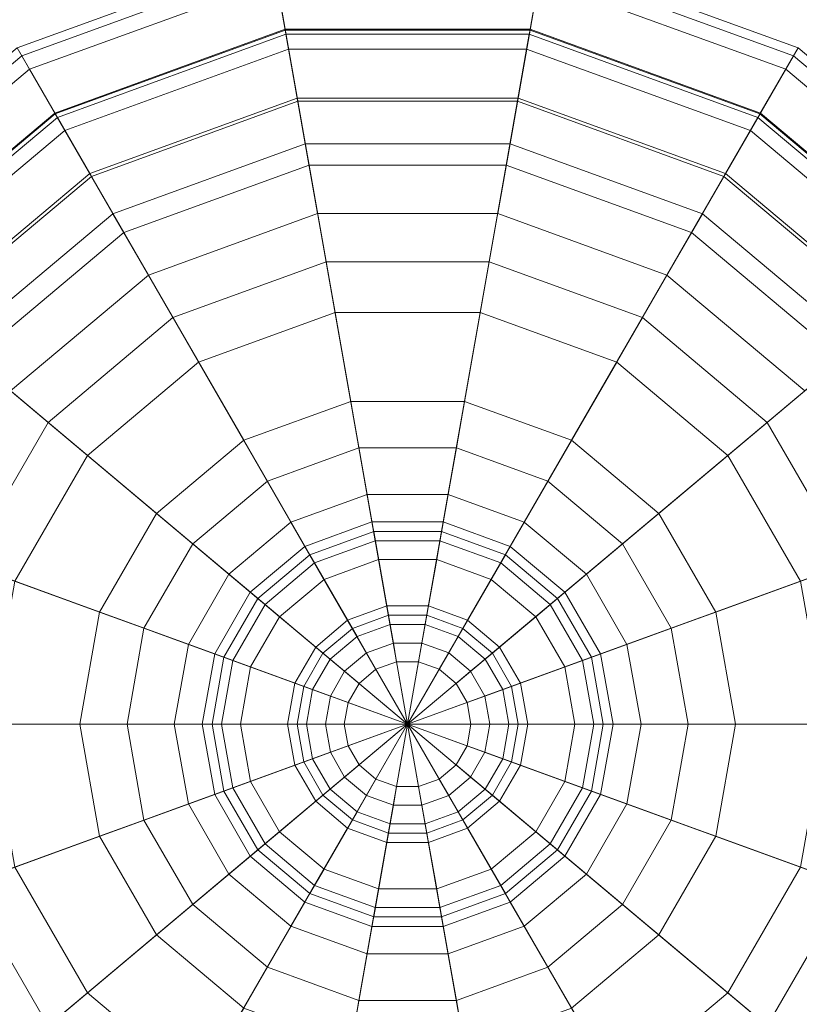
# Model space of a CAD drawing. Units: inches. Extents: x 375 to 1122, y 27 to 1069.
# Tile 32 of 155: x 732.389 to 733.741, y 280.756 to 282.464. Entities that reach past the tile are written whole.
import ezdxf

# ---------------------------------------------------------------- set-up
doc = ezdxf.new("R2010")
doc.units = ezdxf.units.IN
doc.layers.add('A-ANNO-DIMS', color=2, linetype='Continuous', lineweight=18)
doc.layers.add('Furniture', color=30, linetype='Continuous', lineweight=18)
doc.styles.get("Standard").update_dxf_attribs({"font": 'arial.ttf'})
doc.dimstyles.new('ISO-25', dxfattribs={"dimtxt": 12, "dimasz": 2.5, "dimexe": 1.5, "dimexo": 1.5, "dimtad": 1, "dimdec": 1, "dimlunit": 3, "dimtxsty": 'Standard', "dimblk": 'ARCHTICK', "dimcen": 2.5, "dimadec": 0, "dimazin": 0, "dimtfac": 1, "dimtdec": 1, "dimtmove": 0, "dimatfit": 3, "dimfxl": 1.5, "dimfxlon": 1, "dimarcsym": 0})

# ---------------------------------------------------------------- blocks, each defined once
blk = doc.blocks.new('A$C403C54AD')
for points in [[(1.626464, 1.23678, -0.04658), (1.626464, 1.202917, -0.043501), (1.626464, 1.202917, -0.043501), (1.614883, 1.234737, -0.04658)], [(1.638046, 1.234737, -0.04658), (1.626464, 1.202917, -0.043501), (1.626464, 1.202917, -0.043501), (1.626464, 1.23678, -0.04658)], [(1.614883, 1.234737, -0.04658), (1.626464, 1.202917, -0.043501), (1.626464, 1.202917, -0.043501), (1.604698, 1.228857, -0.04658)], [(1.64823, 1.228857, -0.04658), (1.626464, 1.202917, -0.043501), (1.626464, 1.202917, -0.043501), (1.638046, 1.234737, -0.04658)], [(1.626464, 1.217132, -0.040074), (1.626464, 1.233514, -0.043349), (1.616, 1.231669, -0.043349), (1.621603, 1.216274, -0.040074)], [(1.631326, 1.216274, -0.040074), (1.636929, 1.231669, -0.043349), (1.626464, 1.233514, -0.043349), (1.626464, 1.217132, -0.040074)], [(1.621603, 1.216274, -0.040074), (1.616, 1.231669, -0.043349), (1.606797, 1.226356, -0.043349), (1.617327, 1.213806, -0.040074)], [(1.635601, 1.213806, -0.040074), (1.646131, 1.226356, -0.043349), (1.636929, 1.231669, -0.043349), (1.631326, 1.216274, -0.040074)], [(1.604698, 1.228857, -0.04658), (1.626464, 1.202917, -0.043501), (1.626464, 1.202917, -0.043501), (1.597139, 1.219849, -0.04658)], [(1.606797, 1.226356, -0.043349), (1.604698, 1.228857, -0.04658), (1.597139, 1.219849, -0.04658), (1.599967, 1.218216, -0.043349)], [(1.65579, 1.219849, -0.04658), (1.626464, 1.202917, -0.043501), (1.626464, 1.202917, -0.043501), (1.64823, 1.228857, -0.04658)], [(1.606823, 1.226325, 0.116404), (1.604954, 1.228552, 0.10318), (1.597484, 1.219649, 0.10318), (1.600002, 1.218195, 0.116404)], [(1.604954, 1.228552, 0.10318), (1.605388, 1.228035, 0.074938), (1.598069, 1.219312, 0.074938), (1.597484, 1.219649, 0.10318)], [(1.617085, 1.228687, 0.056929), (1.619501, 1.222047, 0.046697), (1.613379, 1.218512, 0.046697), (1.608836, 1.223925, 0.056929)], [(1.644092, 1.223925, 0.056929), (1.63955, 1.218512, 0.046697), (1.633427, 1.222047, 0.046697), (1.635844, 1.228687, 0.056929)], [(1.605388, 1.228035, 0.074938), (1.608836, 1.223925, 0.056929), (1.602714, 1.216629, 0.056929), (1.598069, 1.219312, 0.074938)], [(1.617327, 1.213806, -0.040074), (1.606797, 1.226356, -0.043349), (1.599967, 1.218216, -0.043349), (1.614154, 1.210025, -0.040074)], [(1.610035, 1.222497, 0.12581), (1.606823, 1.226325, 0.116404), (1.600002, 1.218195, 0.116404), (1.604329, 1.215697, 0.12581)], [(1.606937, 1.226189, 0.102963), (1.608743, 1.224037, 0.115599), (1.602589, 1.216702, 0.115599), (1.600155, 1.218107, 0.102963)], [(1.60736, 1.225685, 0.075423), (1.606937, 1.226189, 0.102963), (1.600155, 1.218107, 0.102963), (1.600725, 1.217778, 0.075423)], [(1.638774, 1.210025, -0.040074), (1.652961, 1.218216, -0.043349), (1.646131, 1.226356, -0.043349), (1.635601, 1.213806, -0.040074)], [(1.620264, 1.219951, 0.048884), (1.618046, 1.226046, 0.058276), (1.610643, 1.221772, 0.058276), (1.614812, 1.216804, 0.048884)], [(1.638116, 1.216804, 0.048884), (1.642285, 1.221772, 0.058276), (1.634882, 1.226046, 0.058276), (1.632664, 1.219951, 0.048884)], [(1.610643, 1.221772, 0.058276), (1.60736, 1.225685, 0.075423), (1.600725, 1.217778, 0.075423), (1.605149, 1.215224, 0.058276)], [(1.608743, 1.224037, 0.115599), (1.612014, 1.220139, 0.12581), (1.606995, 1.214158, 0.12581), (1.602589, 1.216702, 0.115599)], [(1.608836, 1.223925, 0.056929), (1.613379, 1.218512, 0.046697), (1.608834, 1.213096, 0.046697), (1.602714, 1.216629, 0.056929)], [(1.626464, 1.223275, 0.046697), (1.626464, 1.213036, 0.03933), (1.623003, 1.212426, 0.03933), (1.619501, 1.222047, 0.046697)], [(1.633427, 1.222047, 0.046697), (1.629925, 1.212426, 0.03933), (1.626464, 1.213036, 0.03933), (1.626464, 1.223275, 0.046697)], [(1.612014, 1.220139, 0.12581), (1.610035, 1.222497, 0.12581), (1.604329, 1.215697, 0.12581), (1.606995, 1.214158, 0.12581)], [(1.619501, 1.222047, 0.046697), (1.623003, 1.212426, 0.03933), (1.61996, 1.210669, 0.03933), (1.613379, 1.218512, 0.046697)], [(1.63955, 1.218512, 0.046697), (1.632968, 1.210669, 0.03933), (1.629925, 1.212426, 0.03933), (1.633427, 1.222047, 0.046697)], [(1.614812, 1.216804, 0.048884), (1.610643, 1.221772, 0.058276), (1.605149, 1.215224, 0.058276), (1.610766, 1.211981, 0.048884)], [(1.642163, 1.211981, 0.048884), (1.64778, 1.215224, 0.058276), (1.642285, 1.221772, 0.058276), (1.638116, 1.216804, 0.048884)], [(1.626464, 1.211822, 0.042248), (1.626464, 1.221045, 0.048884), (1.620264, 1.219951, 0.048884), (1.623419, 1.211285, 0.042248)], [(1.62951, 1.211285, 0.042248), (1.632664, 1.219951, 0.048884), (1.626464, 1.221045, 0.048884), (1.626464, 1.211822, 0.042248)], [(1.597139, 1.219849, -0.04658), (1.626464, 1.202917, -0.043501), (1.626464, 1.202917, -0.043501), (1.593116, 1.208798, -0.04658)], [(1.599967, 1.218216, -0.043349), (1.597139, 1.219849, -0.04658), (1.593116, 1.208798, -0.04658), (1.596333, 1.20823, -0.043349)], [(1.623419, 1.211285, 0.042248), (1.620264, 1.219951, 0.048884), (1.614812, 1.216804, 0.048884), (1.620741, 1.209738, 0.042248)], [(1.659812, 1.208798, -0.04658), (1.626464, 1.202917, -0.043501), (1.626464, 1.202917, -0.043501), (1.65579, 1.219849, -0.04658)], [(1.632188, 1.209738, 0.042248), (1.638116, 1.216804, 0.048884), (1.632664, 1.219951, 0.048884), (1.62951, 1.211285, 0.042248)], [(1.600002, 1.218195, 0.116404), (1.597484, 1.219649, 0.10318), (1.593509, 1.208728, 0.10318), (1.596372, 1.208223, 0.116404)], [(1.597484, 1.219649, 0.10318), (1.598069, 1.219312, 0.074938), (1.594174, 1.208611, 0.074938), (1.593509, 1.208728, 0.10318)], [(1.598069, 1.219312, 0.074938), (1.602714, 1.216629, 0.056929), (1.599457, 1.20768, 0.056929), (1.594174, 1.208611, 0.074938)], [(1.613379, 1.218512, 0.046697), (1.61996, 1.210669, 0.03933), (1.617701, 1.207977, 0.03933), (1.608834, 1.213096, 0.046697)], [(1.644094, 1.213096, 0.046697), (1.635227, 1.207977, 0.03933), (1.632968, 1.210669, 0.03933), (1.63955, 1.218512, 0.046697)], [(1.614154, 1.210025, -0.040074), (1.599967, 1.218216, -0.043349), (1.596333, 1.20823, -0.043349), (1.612466, 1.205386, -0.040074)], [(1.604329, 1.215697, 0.12581), (1.600002, 1.218195, 0.116404), (1.596372, 1.208223, 0.116404), (1.601293, 1.207356, 0.12581)], [(1.600155, 1.218107, 0.102963), (1.602589, 1.216702, 0.115599), (1.599314, 1.207705, 0.115599), (1.596547, 1.208193, 0.102963)], [(1.600725, 1.217778, 0.075423), (1.600155, 1.218107, 0.102963), (1.596547, 1.208193, 0.102963), (1.597195, 1.208078, 0.075423)], [(1.605149, 1.215224, 0.058276), (1.600725, 1.217778, 0.075423), (1.597195, 1.208078, 0.075423), (1.602225, 1.207191, 0.058276)], [(1.620741, 1.209738, 0.042248), (1.614812, 1.216804, 0.048884), (1.610766, 1.211981, 0.048884), (1.618753, 1.207369, 0.042248)], [(1.626464, 1.215084, -0.037209), (1.626464, 1.217132, -0.040074), (1.621603, 1.216274, -0.040074), (1.622303, 1.21435, -0.037209)], [(1.630625, 1.21435, -0.037209), (1.631326, 1.216274, -0.040074), (1.626464, 1.217132, -0.040074), (1.626464, 1.215084, -0.037209)], [(1.634175, 1.207369, 0.042248), (1.642163, 1.211981, 0.048884), (1.638116, 1.216804, 0.048884), (1.632188, 1.209738, 0.042248)], [(1.602589, 1.216702, 0.115599), (1.606995, 1.214158, 0.12581), (1.604324, 1.206821, 0.12581), (1.599314, 1.207705, 0.115599)], [(1.602714, 1.216629, 0.056929), (1.608834, 1.213096, 0.046697), (1.606416, 1.206452, 0.046697), (1.599457, 1.20768, 0.056929)], [(1.622303, 1.21435, -0.037209), (1.621603, 1.216274, -0.040074), (1.617327, 1.213806, -0.040074), (1.618644, 1.212238, -0.037209)], [(1.634285, 1.212238, -0.037209), (1.635601, 1.213806, -0.040074), (1.631326, 1.216274, -0.040074), (1.630625, 1.21435, -0.037209)], [(1.606995, 1.214158, 0.12581), (1.604329, 1.215697, 0.12581), (1.601293, 1.207356, 0.12581), (1.604324, 1.206821, 0.12581)], [(1.610766, 1.211981, 0.048884), (1.605149, 1.215224, 0.058276), (1.602225, 1.207191, 0.058276), (1.608612, 1.206065, 0.048884)], [(1.626464, 1.210988, -0.035163), (1.626464, 1.215084, -0.037209), (1.622303, 1.21435, -0.037209), (1.623704, 1.210502, -0.035163)], [(1.629225, 1.210502, -0.035163), (1.630625, 1.21435, -0.037209), (1.626464, 1.215084, -0.037209), (1.626464, 1.210988, -0.035163)], [(1.623704, 1.210502, -0.035163), (1.622303, 1.21435, -0.037209), (1.618644, 1.212238, -0.037209), (1.621276, 1.2091, -0.035163)], [(1.631652, 1.2091, -0.035163), (1.634285, 1.212238, -0.037209), (1.630625, 1.21435, -0.037209), (1.629225, 1.210502, -0.035163)], [(1.618644, 1.212238, -0.037209), (1.617327, 1.213806, -0.040074), (1.614154, 1.210025, -0.040074), (1.615928, 1.209001, -0.037209)], [(1.637001, 1.209001, -0.037209), (1.638774, 1.210025, -0.040074), (1.635601, 1.213806, -0.040074), (1.634285, 1.212238, -0.037209)], [(1.608834, 1.213096, 0.046697), (1.617701, 1.207977, 0.03933), (1.616499, 1.204675, 0.03933), (1.606416, 1.206452, 0.046697)], [(1.626464, 1.213036, 0.03933), (1.626464, 1.208122, 0.038511), (1.624684, 1.207808, 0.038511), (1.623003, 1.212426, 0.03933)], [(1.629925, 1.212426, 0.03933), (1.628244, 1.207808, 0.038511), (1.626464, 1.208122, 0.038511), (1.626464, 1.213036, 0.03933)], [(1.646512, 1.206452, 0.046697), (1.636429, 1.204675, 0.03933), (1.635227, 1.207977, 0.03933), (1.644094, 1.213096, 0.046697)], [(1.621276, 1.2091, -0.035163), (1.618644, 1.212238, -0.037209), (1.615928, 1.209001, -0.037209), (1.619474, 1.206953, -0.035163)], [(1.623003, 1.212426, 0.03933), (1.624684, 1.207808, 0.038511), (1.623119, 1.206904, 0.038511), (1.61996, 1.210669, 0.03933)], [(1.632968, 1.210669, 0.03933), (1.629809, 1.206904, 0.038511), (1.628244, 1.207808, 0.038511), (1.629925, 1.212426, 0.03933)], [(1.633454, 1.206953, -0.035163), (1.637001, 1.209001, -0.037209), (1.634285, 1.212238, -0.037209), (1.631652, 1.2091, -0.035163)], [(1.618753, 1.207369, 0.042248), (1.610766, 1.211981, 0.048884), (1.608612, 1.206065, 0.048884), (1.617695, 1.204464, 0.042248)], [(1.626464, 1.202917, 0.040765), (1.626464, 1.211822, 0.042248), (1.623419, 1.211285, 0.042248), (1.626464, 1.202917, 0.040765)], [(1.626464, 1.202917, 0.040765), (1.62951, 1.211285, 0.042248), (1.626464, 1.211822, 0.042248), (1.626464, 1.202917, 0.040765)], [(1.635233, 1.204464, 0.042248), (1.644316, 1.206065, 0.048884), (1.642163, 1.211981, 0.048884), (1.634175, 1.207369, 0.042248)], [(1.626464, 1.202917, 0.040765), (1.623419, 1.211285, 0.042248), (1.620741, 1.209738, 0.042248), (1.626464, 1.202917, 0.040765)], [(1.626464, 1.211398, 0.035646), (1.626464, 1.207302, 0.033599), (1.624964, 1.207038, 0.033599), (1.623564, 1.210887, 0.035646)], [(1.626464, 1.210169, 0.037692), (1.626464, 1.211398, 0.035646), (1.623564, 1.210887, 0.035646), (1.623984, 1.209732, 0.037692)], [(1.629365, 1.210887, 0.035646), (1.627964, 1.207038, 0.033599), (1.626464, 1.207302, 0.033599), (1.626464, 1.211398, 0.035646)], [(1.628944, 1.209732, 0.037692), (1.629365, 1.210887, 0.035646), (1.626464, 1.211398, 0.035646), (1.626464, 1.210169, 0.037692)], [(1.626464, 1.202917, 0.040765), (1.632188, 1.209738, 0.042248), (1.62951, 1.211285, 0.042248), (1.626464, 1.202917, 0.040765)], [(1.623564, 1.210887, 0.035646), (1.624964, 1.207038, 0.033599), (1.623646, 1.206277, 0.033599), (1.621013, 1.209414, 0.035646)], [(1.623984, 1.209732, 0.037692), (1.623564, 1.210887, 0.035646), (1.621013, 1.209414, 0.035646), (1.621803, 1.208473, 0.037692)], [(1.626464, 1.207712, -0.029842), (1.626464, 1.210988, -0.035163), (1.623704, 1.210502, -0.035163), (1.624824, 1.207423, -0.029842)], [(1.628104, 1.207423, -0.029842), (1.629225, 1.210502, -0.035163), (1.626464, 1.210988, -0.035163), (1.626464, 1.207712, -0.029842)], [(1.631915, 1.209414, 0.035646), (1.629283, 1.206277, 0.033599), (1.627964, 1.207038, 0.033599), (1.629365, 1.210887, 0.035646)], [(1.631126, 1.208473, 0.037692), (1.631915, 1.209414, 0.035646), (1.629365, 1.210887, 0.035646), (1.628944, 1.209732, 0.037692)], [(1.61996, 1.210669, 0.03933), (1.623119, 1.206904, 0.038511), (1.621957, 1.205519, 0.038511), (1.617701, 1.207977, 0.03933)], [(1.624824, 1.207423, -0.029842), (1.623704, 1.210502, -0.035163), (1.621276, 1.2091, -0.035163), (1.623382, 1.20659, -0.029842)], [(1.629546, 1.20659, -0.029842), (1.631652, 1.2091, -0.035163), (1.629225, 1.210502, -0.035163), (1.628104, 1.207423, -0.029842)], [(1.635227, 1.207977, 0.03933), (1.630971, 1.205519, 0.038511), (1.629809, 1.206904, 0.038511), (1.632968, 1.210669, 0.03933)], [(1.615928, 1.209001, -0.037209), (1.614154, 1.210025, -0.040074), (1.612466, 1.205386, -0.040074), (1.614482, 1.20503, -0.037209)], [(1.626464, 1.208122, 0.038511), (1.626464, 1.210169, 0.037692), (1.623984, 1.209732, 0.037692), (1.624684, 1.207808, 0.038511)], [(1.628244, 1.207808, 0.038511), (1.628944, 1.209732, 0.037692), (1.626464, 1.210169, 0.037692), (1.626464, 1.208122, 0.038511)], [(1.638446, 1.20503, -0.037209), (1.640462, 1.205386, -0.040074), (1.638774, 1.210025, -0.040074), (1.637001, 1.209001, -0.037209)], [(1.626464, 1.202917, 0.040765), (1.620741, 1.209738, 0.042248), (1.618753, 1.207369, 0.042248), (1.626464, 1.202917, 0.040765)], [(1.624684, 1.207808, 0.038511), (1.623984, 1.209732, 0.037692), (1.621803, 1.208473, 0.037692), (1.623119, 1.206904, 0.038511)], [(1.626464, 1.202917, 0.040765), (1.634175, 1.207369, 0.042248), (1.632188, 1.209738, 0.042248), (1.626464, 1.202917, 0.040765)], [(1.629809, 1.206904, 0.038511), (1.631126, 1.208473, 0.037692), (1.628944, 1.209732, 0.037692), (1.628244, 1.207808, 0.038511)], [(1.621013, 1.209414, 0.035646), (1.623646, 1.206277, 0.033599), (1.622667, 1.20511, 0.033599), (1.61912, 1.207158, 0.035646)], [(1.621803, 1.208473, 0.037692), (1.621013, 1.209414, 0.035646), (1.61912, 1.207158, 0.035646), (1.620184, 1.206543, 0.037692)], [(1.623382, 1.20659, -0.029842), (1.621276, 1.2091, -0.035163), (1.619474, 1.206953, -0.035163), (1.622312, 1.205315, -0.029842)], [(1.633809, 1.207158, 0.035646), (1.630262, 1.20511, 0.033599), (1.629283, 1.206277, 0.033599), (1.631915, 1.209414, 0.035646)], [(1.630616, 1.205315, -0.029842), (1.633454, 1.206953, -0.035163), (1.631652, 1.2091, -0.035163), (1.629546, 1.20659, -0.029842)], [(1.632744, 1.206543, 0.037692), (1.633809, 1.207158, 0.035646), (1.631915, 1.209414, 0.035646), (1.631126, 1.208473, 0.037692)], [(1.593116, 1.208798, -0.04658), (1.626464, 1.202917, -0.043501), (1.626464, 1.202917, -0.043501), (1.593116, 1.197037, -0.04658)], [(1.596333, 1.20823, -0.043349), (1.593116, 1.208798, -0.04658), (1.593116, 1.197037, -0.04658), (1.596333, 1.197604, -0.043349)], [(1.596372, 1.208223, 0.116404), (1.593509, 1.208728, 0.10318), (1.593509, 1.197107, 0.10318), (1.596372, 1.197611, 0.116404)], [(1.619474, 1.206953, -0.035163), (1.615928, 1.209001, -0.037209), (1.614482, 1.20503, -0.037209), (1.618516, 1.204319, -0.035163)], [(1.659812, 1.197037, -0.04658), (1.626464, 1.202917, -0.043501), (1.626464, 1.202917, -0.043501), (1.659812, 1.208798, -0.04658)], [(1.634413, 1.204319, -0.035163), (1.638446, 1.20503, -0.037209), (1.637001, 1.209001, -0.037209), (1.633454, 1.206953, -0.035163)], [(1.594174, 1.208611, 0.074938), (1.599457, 1.20768, 0.056929), (1.599457, 1.198155, 0.056929), (1.594174, 1.197224, 0.074938)], [(1.623119, 1.206904, 0.038511), (1.621803, 1.208473, 0.037692), (1.620184, 1.206543, 0.037692), (1.621957, 1.205519, 0.038511)], [(1.630971, 1.205519, 0.038511), (1.632744, 1.206543, 0.037692), (1.631126, 1.208473, 0.037692), (1.629809, 1.206904, 0.038511)], [(1.612466, 1.205386, -0.040074), (1.596333, 1.20823, -0.043349), (1.596333, 1.197604, -0.043349), (1.612466, 1.200449, -0.040074)], [(1.601293, 1.207356, 0.12581), (1.596372, 1.208223, 0.116404), (1.596372, 1.197611, 0.116404), (1.601293, 1.198479, 0.12581)], [(1.596547, 1.208193, 0.102963), (1.599314, 1.207705, 0.115599), (1.599314, 1.19813, 0.115599), (1.596547, 1.197642, 0.102963)], [(1.597195, 1.208078, 0.075423), (1.596547, 1.208193, 0.102963), (1.596547, 1.197642, 0.102963), (1.597195, 1.197756, 0.075423)], [(1.602225, 1.207191, 0.058276), (1.597195, 1.208078, 0.075423), (1.597195, 1.197756, 0.075423), (1.602225, 1.198643, 0.058276)], [(1.617701, 1.207977, 0.03933), (1.621957, 1.205519, 0.038511), (1.621339, 1.203821, 0.038511), (1.616499, 1.204675, 0.03933)], [(1.636429, 1.204675, 0.03933), (1.631589, 1.203821, 0.038511), (1.630971, 1.205519, 0.038511), (1.635227, 1.207977, 0.03933)], [(1.599314, 1.207705, 0.115599), (1.604324, 1.206821, 0.12581), (1.604324, 1.199014, 0.12581), (1.599314, 1.19813, 0.115599)], [(1.599457, 1.20768, 0.056929), (1.606416, 1.206452, 0.046697), (1.606416, 1.199382, 0.046697), (1.599457, 1.198155, 0.056929)], [(1.625245, 1.206268, -0.021247), (1.624824, 1.207423, -0.029842), (1.623382, 1.20659, -0.029842), (1.624172, 1.205649, -0.021247)], [(1.626464, 1.206483, -0.021247), (1.626464, 1.207712, -0.029842), (1.624824, 1.207423, -0.029842), (1.625245, 1.206268, -0.021247)], [(1.627684, 1.206268, -0.021247), (1.628104, 1.207423, -0.029842), (1.626464, 1.207712, -0.029842), (1.626464, 1.206483, -0.021247)], [(1.628756, 1.205649, -0.021247), (1.629546, 1.20659, -0.029842), (1.628104, 1.207423, -0.029842), (1.627684, 1.206268, -0.021247)], [(1.604324, 1.206821, 0.12581), (1.601293, 1.207356, 0.12581), (1.601293, 1.198479, 0.12581), (1.604324, 1.199014, 0.12581)], [(1.608612, 1.206065, 0.048884), (1.602225, 1.207191, 0.058276), (1.602225, 1.198643, 0.058276), (1.608612, 1.19977, 0.048884)], [(1.626464, 1.202917, 0.040765), (1.618753, 1.207369, 0.042248), (1.617695, 1.204464, 0.042248), (1.626464, 1.202917, 0.040765)], [(1.61912, 1.207158, 0.035646), (1.622667, 1.20511, 0.033599), (1.622146, 1.203679, 0.033599), (1.618112, 1.20439, 0.035646)], [(1.620184, 1.206543, 0.037692), (1.61912, 1.207158, 0.035646), (1.618112, 1.20439, 0.035646), (1.619322, 1.204177, 0.037692)], [(1.622312, 1.205315, -0.029842), (1.619474, 1.206953, -0.035163), (1.618516, 1.204319, -0.035163), (1.621742, 1.20375, -0.029842)], [(1.624964, 1.207038, 0.033599), (1.625525, 1.205499, 0.027051), (1.624699, 1.205022, 0.027051), (1.623646, 1.206277, 0.033599)], [(1.626464, 1.207302, 0.033599), (1.626464, 1.205664, 0.027051), (1.625525, 1.205499, 0.027051), (1.624964, 1.207038, 0.033599)], [(1.626464, 1.202917, 0.040765), (1.635233, 1.204464, 0.042248), (1.634175, 1.207369, 0.042248), (1.626464, 1.202917, 0.040765)], [(1.627964, 1.207038, 0.033599), (1.627404, 1.205499, 0.027051), (1.626464, 1.205664, 0.027051), (1.626464, 1.207302, 0.033599)], [(1.629283, 1.206277, 0.033599), (1.62823, 1.205022, 0.027051), (1.627404, 1.205499, 0.027051), (1.627964, 1.207038, 0.033599)], [(1.634816, 1.20439, 0.035646), (1.630783, 1.203679, 0.033599), (1.630262, 1.20511, 0.033599), (1.633809, 1.207158, 0.035646)], [(1.631186, 1.20375, -0.029842), (1.634413, 1.204319, -0.035163), (1.633454, 1.206953, -0.035163), (1.630616, 1.205315, -0.029842)], [(1.633606, 1.204177, 0.037692), (1.634816, 1.20439, 0.035646), (1.633809, 1.207158, 0.035646), (1.632744, 1.206543, 0.037692)], [(1.621957, 1.205519, 0.038511), (1.620184, 1.206543, 0.037692), (1.619322, 1.204177, 0.037692), (1.621339, 1.203821, 0.038511)], [(1.624172, 1.205649, -0.021247), (1.623382, 1.20659, -0.029842), (1.622312, 1.205315, -0.029842), (1.623376, 1.2047, -0.021247)], [(1.629552, 1.2047, -0.021247), (1.630616, 1.205315, -0.029842), (1.629546, 1.20659, -0.029842), (1.628756, 1.205649, -0.021247)], [(1.631589, 1.203821, 0.038511), (1.633606, 1.204177, 0.037692), (1.632744, 1.206543, 0.037692), (1.630971, 1.205519, 0.038511)], [(1.606416, 1.206452, 0.046697), (1.616499, 1.204675, 0.03933), (1.616499, 1.20116, 0.03933), (1.606416, 1.199382, 0.046697)], [(1.623646, 1.206277, 0.033599), (1.624699, 1.205022, 0.027051), (1.624085, 1.204291, 0.027051), (1.622667, 1.20511, 0.033599)], [(1.625525, 1.205499, 0.027051), (1.625245, 1.206268, -0.021247), (1.624172, 1.205649, -0.021247), (1.624699, 1.205022, 0.027051)], [(1.626464, 1.205664, 0.027051), (1.626464, 1.206483, -0.021247), (1.625245, 1.206268, -0.021247), (1.625525, 1.205499, 0.027051)], [(1.627404, 1.205499, 0.027051), (1.627684, 1.206268, -0.021247), (1.626464, 1.206483, -0.021247), (1.626464, 1.205664, 0.027051)], [(1.62823, 1.205022, 0.027051), (1.628756, 1.205649, -0.021247), (1.627684, 1.206268, -0.021247), (1.627404, 1.205499, 0.027051)], [(1.630262, 1.20511, 0.033599), (1.628843, 1.204291, 0.027051), (1.62823, 1.205022, 0.027051), (1.629283, 1.206277, 0.033599)], [(1.646512, 1.199382, 0.046697), (1.636429, 1.20116, 0.03933), (1.636429, 1.204675, 0.03933), (1.646512, 1.206452, 0.046697)], [(1.617695, 1.204464, 0.042248), (1.608612, 1.206065, 0.048884), (1.608612, 1.19977, 0.048884), (1.617695, 1.201371, 0.042248)], [(1.635233, 1.201371, 0.042248), (1.644316, 1.19977, 0.048884), (1.644316, 1.206065, 0.048884), (1.635233, 1.204464, 0.042248)], [(1.614482, 1.20503, -0.037209), (1.612466, 1.205386, -0.040074), (1.612466, 1.200449, -0.040074), (1.614482, 1.200805, -0.037209)], [(1.623376, 1.2047, -0.021247), (1.622312, 1.205315, -0.029842), (1.621742, 1.20375, -0.029842), (1.622952, 1.203537, -0.021247)], [(1.624699, 1.205022, 0.027051), (1.624172, 1.205649, -0.021247), (1.623376, 1.2047, -0.021247), (1.624085, 1.204291, 0.027051)], [(1.628843, 1.204291, 0.027051), (1.629552, 1.2047, -0.021247), (1.628756, 1.205649, -0.021247), (1.62823, 1.205022, 0.027051)], [(1.629976, 1.203537, -0.021247), (1.631186, 1.20375, -0.029842), (1.630616, 1.205315, -0.029842), (1.629552, 1.2047, -0.021247)], [(1.638446, 1.200805, -0.037209), (1.640462, 1.200449, -0.040074), (1.640462, 1.205386, -0.040074), (1.638446, 1.20503, -0.037209)], [(1.618516, 1.204319, -0.035163), (1.614482, 1.20503, -0.037209), (1.614482, 1.200805, -0.037209), (1.618516, 1.201516, -0.035163)], [(1.622667, 1.20511, 0.033599), (1.624085, 1.204291, 0.027051), (1.623759, 1.203394, 0.027051), (1.622146, 1.203679, 0.033599)], [(1.630783, 1.203679, 0.033599), (1.629169, 1.203394, 0.027051), (1.628843, 1.204291, 0.027051), (1.630262, 1.20511, 0.033599)], [(1.634413, 1.201516, -0.035163), (1.638446, 1.200805, -0.037209), (1.638446, 1.20503, -0.037209), (1.634413, 1.204319, -0.035163)], [(1.616499, 1.204675, 0.03933), (1.621339, 1.203821, 0.038511), (1.621339, 1.202014, 0.038511), (1.616499, 1.20116, 0.03933)], [(1.626464, 1.202917, 0.040765), (1.617695, 1.204464, 0.042248), (1.617695, 1.201371, 0.042248), (1.626464, 1.202917, 0.040765)], [(1.618112, 1.20439, 0.035646), (1.622146, 1.203679, 0.033599), (1.622146, 1.202156, 0.033599), (1.618112, 1.201445, 0.035646)], [(1.619322, 1.204177, 0.037692), (1.618112, 1.20439, 0.035646), (1.618112, 1.201445, 0.035646), (1.619322, 1.201658, 0.037692)], [(1.624085, 1.204291, 0.027051), (1.623376, 1.2047, -0.021247), (1.622952, 1.203537, -0.021247), (1.623759, 1.203394, 0.027051)], [(1.626464, 1.202917, 0.040765), (1.635233, 1.201371, 0.042248), (1.635233, 1.204464, 0.042248), (1.626464, 1.202917, 0.040765)], [(1.629169, 1.203394, 0.027051), (1.629976, 1.203537, -0.021247), (1.629552, 1.2047, -0.021247), (1.628843, 1.204291, 0.027051)], [(1.634816, 1.201445, 0.035646), (1.630783, 1.202156, 0.033599), (1.630783, 1.203679, 0.033599), (1.634816, 1.20439, 0.035646)], [(1.636429, 1.20116, 0.03933), (1.631589, 1.202014, 0.038511), (1.631589, 1.203821, 0.038511), (1.636429, 1.204675, 0.03933)], [(1.633606, 1.201658, 0.037692), (1.634816, 1.201445, 0.035646), (1.634816, 1.20439, 0.035646), (1.633606, 1.204177, 0.037692)], [(1.621742, 1.20375, -0.029842), (1.618516, 1.204319, -0.035163), (1.618516, 1.201516, -0.035163), (1.621742, 1.202085, -0.029842)], [(1.621339, 1.203821, 0.038511), (1.619322, 1.204177, 0.037692), (1.619322, 1.201658, 0.037692), (1.621339, 1.202014, 0.038511)], [(1.631186, 1.202085, -0.029842), (1.634413, 1.201516, -0.035163), (1.634413, 1.204319, -0.035163), (1.631186, 1.20375, -0.029842)], [(1.631589, 1.202014, 0.038511), (1.633606, 1.201658, 0.037692), (1.633606, 1.204177, 0.037692), (1.631589, 1.203821, 0.038511)], [(1.622952, 1.203537, -0.021247), (1.621742, 1.20375, -0.029842), (1.621742, 1.202085, -0.029842), (1.622952, 1.202298, -0.021247)], [(1.622146, 1.203679, 0.033599), (1.623759, 1.203394, 0.027051), (1.623759, 1.20244, 0.027051), (1.622146, 1.202156, 0.033599)], [(1.623759, 1.203394, 0.027051), (1.622952, 1.203537, -0.021247), (1.622952, 1.202298, -0.021247), (1.623759, 1.20244, 0.027051)], [(1.630783, 1.202156, 0.033599), (1.629169, 1.20244, 0.027051), (1.629169, 1.203394, 0.027051), (1.630783, 1.203679, 0.033599)], [(1.629169, 1.20244, 0.027051), (1.629976, 1.202298, -0.021247), (1.629976, 1.203537, -0.021247), (1.629169, 1.203394, 0.027051)], [(1.629976, 1.202298, -0.021247), (1.631186, 1.202085, -0.029842), (1.631186, 1.20375, -0.029842), (1.629976, 1.203537, -0.021247)], [(1.593116, 1.197037, -0.04658), (1.626464, 1.202917, -0.043501), (1.626464, 1.202917, -0.043501), (1.597139, 1.185986, -0.04658)], [(1.597139, 1.185986, -0.04658), (1.626464, 1.202917, -0.043501), (1.626464, 1.202917, -0.043501), (1.604698, 1.176977, -0.04658)], [(1.604698, 1.176977, -0.04658), (1.626464, 1.202917, -0.043501), (1.626464, 1.202917, -0.043501), (1.614883, 1.171097, -0.04658)], [(1.614883, 1.171097, -0.04658), (1.626464, 1.202917, -0.043501), (1.626464, 1.202917, -0.043501), (1.626464, 1.169055, -0.04658)], [(1.626464, 1.202917, 0.040765), (1.617695, 1.201371, 0.042248), (1.618753, 1.198465, 0.042248), (1.626464, 1.202917, 0.040765)], [(1.626464, 1.202917, 0.040765), (1.618753, 1.198465, 0.042248), (1.620741, 1.196096, 0.042248), (1.626464, 1.202917, 0.040765)], [(1.626464, 1.202917, 0.040765), (1.620741, 1.196096, 0.042248), (1.623419, 1.19455, 0.042248), (1.626464, 1.202917, 0.040765)], [(1.626464, 1.202917, 0.040765), (1.623419, 1.19455, 0.042248), (1.626464, 1.194013, 0.042248), (1.626464, 1.202917, 0.040765)], [(1.626464, 1.202917, 0.040765), (1.62951, 1.19455, 0.042248), (1.632188, 1.196096, 0.042248), (1.626464, 1.202917, 0.040765)], [(1.626464, 1.202917, 0.040765), (1.626464, 1.194013, 0.042248), (1.62951, 1.19455, 0.042248), (1.626464, 1.202917, 0.040765)], [(1.626464, 1.202917, 0.040765), (1.634175, 1.198465, 0.042248), (1.635233, 1.201371, 0.042248), (1.626464, 1.202917, 0.040765)], [(1.626464, 1.202917, 0.040765), (1.632188, 1.196096, 0.042248), (1.634175, 1.198465, 0.042248), (1.626464, 1.202917, 0.040765)], [(1.65579, 1.185986, -0.04658), (1.626464, 1.202917, -0.043501), (1.626464, 1.202917, -0.043501), (1.659812, 1.197037, -0.04658)], [(1.64823, 1.176977, -0.04658), (1.626464, 1.202917, -0.043501), (1.626464, 1.202917, -0.043501), (1.65579, 1.185986, -0.04658)], [(1.638046, 1.171097, -0.04658), (1.626464, 1.202917, -0.043501), (1.626464, 1.202917, -0.043501), (1.64823, 1.176977, -0.04658)], [(1.626464, 1.169055, -0.04658), (1.626464, 1.202917, -0.043501), (1.626464, 1.202917, -0.043501), (1.638046, 1.171097, -0.04658)], [(1.622952, 1.202298, -0.021247), (1.621742, 1.202085, -0.029842), (1.622312, 1.20052, -0.029842), (1.623376, 1.201134, -0.021247)], [(1.622146, 1.202156, 0.033599), (1.623759, 1.20244, 0.027051), (1.624085, 1.201544, 0.027051), (1.622667, 1.200725, 0.033599)], [(1.623759, 1.20244, 0.027051), (1.622952, 1.202298, -0.021247), (1.623376, 1.201134, -0.021247), (1.624085, 1.201544, 0.027051)], [(1.630262, 1.200725, 0.033599), (1.628843, 1.201544, 0.027051), (1.629169, 1.20244, 0.027051), (1.630783, 1.202156, 0.033599)], [(1.628843, 1.201544, 0.027051), (1.629552, 1.201134, -0.021247), (1.629976, 1.202298, -0.021247), (1.629169, 1.20244, 0.027051)], [(1.629552, 1.201134, -0.021247), (1.630616, 1.20052, -0.029842), (1.631186, 1.202085, -0.029842), (1.629976, 1.202298, -0.021247)], [(1.616499, 1.20116, 0.03933), (1.621339, 1.202014, 0.038511), (1.621957, 1.200315, 0.038511), (1.617701, 1.197858, 0.03933)], [(1.618112, 1.201445, 0.035646), (1.622146, 1.202156, 0.033599), (1.622667, 1.200725, 0.033599), (1.61912, 1.198677, 0.035646)], [(1.621742, 1.202085, -0.029842), (1.618516, 1.201516, -0.035163), (1.619474, 1.198882, -0.035163), (1.622312, 1.20052, -0.029842)], [(1.621339, 1.202014, 0.038511), (1.619322, 1.201658, 0.037692), (1.620184, 1.199291, 0.037692), (1.621957, 1.200315, 0.038511)], [(1.633809, 1.198677, 0.035646), (1.630262, 1.200725, 0.033599), (1.630783, 1.202156, 0.033599), (1.634816, 1.201445, 0.035646)], [(1.630616, 1.20052, -0.029842), (1.633454, 1.198882, -0.035163), (1.634413, 1.201516, -0.035163), (1.631186, 1.202085, -0.029842)], [(1.630971, 1.200315, 0.038511), (1.632744, 1.199291, 0.037692), (1.633606, 1.201658, 0.037692), (1.631589, 1.202014, 0.038511)], [(1.635227, 1.197858, 0.03933), (1.630971, 1.200315, 0.038511), (1.631589, 1.202014, 0.038511), (1.636429, 1.20116, 0.03933)], [(1.618516, 1.201516, -0.035163), (1.614482, 1.200805, -0.037209), (1.615928, 1.196834, -0.037209), (1.619474, 1.198882, -0.035163)], [(1.619322, 1.201658, 0.037692), (1.618112, 1.201445, 0.035646), (1.61912, 1.198677, 0.035646), (1.620184, 1.199291, 0.037692)], [(1.622667, 1.200725, 0.033599), (1.624085, 1.201544, 0.027051), (1.624699, 1.200813, 0.027051), (1.623646, 1.199558, 0.033599)], [(1.624085, 1.201544, 0.027051), (1.623376, 1.201134, -0.021247), (1.624172, 1.200186, -0.021247), (1.624699, 1.200813, 0.027051)], [(1.629283, 1.199558, 0.033599), (1.62823, 1.200813, 0.027051), (1.628843, 1.201544, 0.027051), (1.630262, 1.200725, 0.033599)], [(1.62823, 1.200813, 0.027051), (1.628756, 1.200186, -0.021247), (1.629552, 1.201134, -0.021247), (1.628843, 1.201544, 0.027051)], [(1.632744, 1.199291, 0.037692), (1.633809, 1.198677, 0.035646), (1.634816, 1.201445, 0.035646), (1.633606, 1.201658, 0.037692)], [(1.633454, 1.198882, -0.035163), (1.637001, 1.196834, -0.037209), (1.638446, 1.200805, -0.037209), (1.634413, 1.201516, -0.035163)], [(1.606416, 1.199382, 0.046697), (1.616499, 1.20116, 0.03933), (1.617701, 1.197858, 0.03933), (1.608834, 1.192739, 0.046697)], [(1.617695, 1.201371, 0.042248), (1.608612, 1.19977, 0.048884), (1.610766, 1.193854, 0.048884), (1.618753, 1.198465, 0.042248)], [(1.623376, 1.201134, -0.021247), (1.622312, 1.20052, -0.029842), (1.623382, 1.199245, -0.029842), (1.624172, 1.200186, -0.021247)], [(1.628756, 1.200186, -0.021247), (1.629546, 1.199245, -0.029842), (1.630616, 1.20052, -0.029842), (1.629552, 1.201134, -0.021247)], [(1.634175, 1.198465, 0.042248), (1.642163, 1.193854, 0.048884), (1.644316, 1.19977, 0.048884), (1.635233, 1.201371, 0.042248)], [(1.644094, 1.192739, 0.046697), (1.635227, 1.197858, 0.03933), (1.636429, 1.20116, 0.03933), (1.646512, 1.199382, 0.046697)], [(1.614482, 1.200805, -0.037209), (1.612466, 1.200449, -0.040074), (1.614154, 1.19581, -0.040074), (1.615928, 1.196834, -0.037209)], [(1.61912, 1.198677, 0.035646), (1.622667, 1.200725, 0.033599), (1.623646, 1.199558, 0.033599), (1.621013, 1.196421, 0.035646)], [(1.623646, 1.199558, 0.033599), (1.624699, 1.200813, 0.027051), (1.625525, 1.200336, 0.027051), (1.624964, 1.198797, 0.033599)], [(1.624699, 1.200813, 0.027051), (1.624172, 1.200186, -0.021247), (1.625245, 1.199567, -0.021247), (1.625525, 1.200336, 0.027051)], [(1.627964, 1.198797, 0.033599), (1.627404, 1.200336, 0.027051), (1.62823, 1.200813, 0.027051), (1.629283, 1.199558, 0.033599)], [(1.627404, 1.200336, 0.027051), (1.627684, 1.199567, -0.021247), (1.628756, 1.200186, -0.021247), (1.62823, 1.200813, 0.027051)], [(1.631915, 1.196421, 0.035646), (1.629283, 1.199558, 0.033599), (1.630262, 1.200725, 0.033599), (1.633809, 1.198677, 0.035646)], [(1.637001, 1.196834, -0.037209), (1.638774, 1.19581, -0.040074), (1.640462, 1.200449, -0.040074), (1.638446, 1.200805, -0.037209)], [(1.612466, 1.200449, -0.040074), (1.596333, 1.197604, -0.043349), (1.599967, 1.187619, -0.043349), (1.614154, 1.19581, -0.040074)], [(1.617701, 1.197858, 0.03933), (1.621957, 1.200315, 0.038511), (1.623119, 1.198931, 0.038511), (1.61996, 1.195166, 0.03933)], [(1.622312, 1.20052, -0.029842), (1.619474, 1.198882, -0.035163), (1.621276, 1.196735, -0.035163), (1.623382, 1.199245, -0.029842)], [(1.621957, 1.200315, 0.038511), (1.620184, 1.199291, 0.037692), (1.621803, 1.197362, 0.037692), (1.623119, 1.198931, 0.038511)], [(1.624172, 1.200186, -0.021247), (1.623382, 1.199245, -0.029842), (1.624824, 1.198412, -0.029842), (1.625245, 1.199567, -0.021247)], [(1.624964, 1.198797, 0.033599), (1.625525, 1.200336, 0.027051), (1.626464, 1.200171, 0.027051), (1.626464, 1.198532, 0.033599)], [(1.625525, 1.200336, 0.027051), (1.625245, 1.199567, -0.021247), (1.626464, 1.199352, -0.021247), (1.626464, 1.200171, 0.027051)], [(1.626464, 1.198532, 0.033599), (1.626464, 1.200171, 0.027051), (1.627404, 1.200336, 0.027051), (1.627964, 1.198797, 0.033599)], [(1.626464, 1.200171, 0.027051), (1.626464, 1.199352, -0.021247), (1.627684, 1.199567, -0.021247), (1.627404, 1.200336, 0.027051)], [(1.627684, 1.199567, -0.021247), (1.628104, 1.198412, -0.029842), (1.629546, 1.199245, -0.029842), (1.628756, 1.200186, -0.021247)], [(1.629546, 1.199245, -0.029842), (1.631652, 1.196735, -0.035163), (1.633454, 1.198882, -0.035163), (1.630616, 1.20052, -0.029842)], [(1.629809, 1.198931, 0.038511), (1.631126, 1.197362, 0.037692), (1.632744, 1.199291, 0.037692), (1.630971, 1.200315, 0.038511)], [(1.632968, 1.195166, 0.03933), (1.629809, 1.198931, 0.038511), (1.630971, 1.200315, 0.038511), (1.635227, 1.197858, 0.03933)], [(1.608612, 1.19977, 0.048884), (1.602225, 1.198643, 0.058276), (1.605149, 1.190611, 0.058276), (1.610766, 1.193854, 0.048884)], [(1.599457, 1.198155, 0.056929), (1.606416, 1.199382, 0.046697), (1.608834, 1.192739, 0.046697), (1.602714, 1.189206, 0.056929)], [(1.620184, 1.199291, 0.037692), (1.61912, 1.198677, 0.035646), (1.621013, 1.196421, 0.035646), (1.621803, 1.197362, 0.037692)], [(1.621013, 1.196421, 0.035646), (1.623646, 1.199558, 0.033599), (1.624964, 1.198797, 0.033599), (1.623564, 1.194948, 0.035646)], [(1.625245, 1.199567, -0.021247), (1.624824, 1.198412, -0.029842), (1.626464, 1.198123, -0.029842), (1.626464, 1.199352, -0.021247)], [(1.626464, 1.199352, -0.021247), (1.626464, 1.198123, -0.029842), (1.628104, 1.198412, -0.029842), (1.627684, 1.199567, -0.021247)], [(1.629365, 1.194948, 0.035646), (1.627964, 1.198797, 0.033599), (1.629283, 1.199558, 0.033599), (1.631915, 1.196421, 0.035646)], [(1.631126, 1.197362, 0.037692), (1.631915, 1.196421, 0.035646), (1.633809, 1.198677, 0.035646), (1.632744, 1.199291, 0.037692)], [(1.599314, 1.19813, 0.115599), (1.604324, 1.199014, 0.12581), (1.606995, 1.191677, 0.12581), (1.602589, 1.189133, 0.115599)], [(1.604324, 1.199014, 0.12581), (1.601293, 1.198479, 0.12581), (1.604329, 1.190138, 0.12581), (1.606995, 1.191677, 0.12581)], [(1.619474, 1.198882, -0.035163), (1.615928, 1.196834, -0.037209), (1.618644, 1.193597, -0.037209), (1.621276, 1.196735, -0.035163)], [(1.61996, 1.195166, 0.03933), (1.623119, 1.198931, 0.038511), (1.624684, 1.198027, 0.038511), (1.623003, 1.193409, 0.03933)], [(1.623382, 1.199245, -0.029842), (1.621276, 1.196735, -0.035163), (1.623704, 1.195333, -0.035163), (1.624824, 1.198412, -0.029842)], [(1.623119, 1.198931, 0.038511), (1.621803, 1.197362, 0.037692), (1.623984, 1.196103, 0.037692), (1.624684, 1.198027, 0.038511)], [(1.628104, 1.198412, -0.029842), (1.629225, 1.195333, -0.035163), (1.631652, 1.196735, -0.035163), (1.629546, 1.199245, -0.029842)], [(1.628244, 1.198027, 0.038511), (1.628944, 1.196103, 0.037692), (1.631126, 1.197362, 0.037692), (1.629809, 1.198931, 0.038511)], [(1.629925, 1.193409, 0.03933), (1.628244, 1.198027, 0.038511), (1.629809, 1.198931, 0.038511), (1.632968, 1.195166, 0.03933)], [(1.631652, 1.196735, -0.035163), (1.634285, 1.193597, -0.037209), (1.637001, 1.196834, -0.037209), (1.633454, 1.198882, -0.035163)], [(1.601293, 1.198479, 0.12581), (1.596372, 1.197611, 0.116404), (1.600002, 1.187639, 0.116404), (1.604329, 1.190138, 0.12581)], [(1.602225, 1.198643, 0.058276), (1.597195, 1.197756, 0.075423), (1.600725, 1.188057, 0.075423), (1.605149, 1.190611, 0.058276)], [(1.618753, 1.198465, 0.042248), (1.610766, 1.193854, 0.048884), (1.614812, 1.189031, 0.048884), (1.620741, 1.196096, 0.042248)], [(1.623564, 1.194948, 0.035646), (1.624964, 1.198797, 0.033599), (1.626464, 1.198532, 0.033599), (1.626464, 1.194437, 0.035646)], [(1.624824, 1.198412, -0.029842), (1.623704, 1.195333, -0.035163), (1.626464, 1.194846, -0.035163), (1.626464, 1.198123, -0.029842)], [(1.626464, 1.194437, 0.035646), (1.626464, 1.198532, 0.033599), (1.627964, 1.198797, 0.033599), (1.629365, 1.194948, 0.035646)], [(1.626464, 1.198123, -0.029842), (1.626464, 1.194846, -0.035163), (1.629225, 1.195333, -0.035163), (1.628104, 1.198412, -0.029842)], [(1.632188, 1.196096, 0.042248), (1.638116, 1.189031, 0.048884), (1.642163, 1.193854, 0.048884), (1.634175, 1.198465, 0.042248)], [(1.594174, 1.197224, 0.074938), (1.599457, 1.198155, 0.056929), (1.602714, 1.189206, 0.056929), (1.598069, 1.186523, 0.074938)], [(1.596547, 1.197642, 0.102963), (1.599314, 1.19813, 0.115599), (1.602589, 1.189133, 0.115599), (1.600155, 1.187728, 0.102963)], [(1.623003, 1.193409, 0.03933), (1.624684, 1.198027, 0.038511), (1.626464, 1.197713, 0.038511), (1.626464, 1.192799, 0.03933)], [(1.624684, 1.198027, 0.038511), (1.623984, 1.196103, 0.037692), (1.626464, 1.195666, 0.037692), (1.626464, 1.197713, 0.038511)], [(1.626464, 1.197713, 0.038511), (1.626464, 1.195666, 0.037692), (1.628944, 1.196103, 0.037692), (1.628244, 1.198027, 0.038511)], [(1.626464, 1.192799, 0.03933), (1.626464, 1.197713, 0.038511), (1.628244, 1.198027, 0.038511), (1.629925, 1.193409, 0.03933)], [(1.596333, 1.197604, -0.043349), (1.593116, 1.197037, -0.04658), (1.597139, 1.185986, -0.04658), (1.599967, 1.187619, -0.043349)], [(1.596372, 1.197611, 0.116404), (1.593509, 1.197107, 0.10318), (1.597484, 1.186186, 0.10318), (1.600002, 1.187639, 0.116404)], [(1.597195, 1.197756, 0.075423), (1.596547, 1.197642, 0.102963), (1.600155, 1.187728, 0.102963), (1.600725, 1.188057, 0.075423)], [(1.608834, 1.192739, 0.046697), (1.617701, 1.197858, 0.03933), (1.61996, 1.195166, 0.03933), (1.613379, 1.187323, 0.046697)], [(1.63955, 1.187323, 0.046697), (1.632968, 1.195166, 0.03933), (1.635227, 1.197858, 0.03933), (1.644094, 1.192739, 0.046697)], [(1.593509, 1.197107, 0.10318), (1.594174, 1.197224, 0.074938), (1.598069, 1.186523, 0.074938), (1.597484, 1.186186, 0.10318)], [(1.621803, 1.197362, 0.037692), (1.621013, 1.196421, 0.035646), (1.623564, 1.194948, 0.035646), (1.623984, 1.196103, 0.037692)], [(1.628944, 1.196103, 0.037692), (1.629365, 1.194948, 0.035646), (1.631915, 1.196421, 0.035646), (1.631126, 1.197362, 0.037692)], [(1.615928, 1.196834, -0.037209), (1.614154, 1.19581, -0.040074), (1.617327, 1.192029, -0.040074), (1.618644, 1.193597, -0.037209)], [(1.621276, 1.196735, -0.035163), (1.618644, 1.193597, -0.037209), (1.622303, 1.191485, -0.037209), (1.623704, 1.195333, -0.035163)], [(1.629225, 1.195333, -0.035163), (1.630625, 1.191485, -0.037209), (1.634285, 1.193597, -0.037209), (1.631652, 1.196735, -0.035163)], [(1.634285, 1.193597, -0.037209), (1.635601, 1.192029, -0.040074), (1.638774, 1.19581, -0.040074), (1.637001, 1.196834, -0.037209)], [(1.620741, 1.196096, 0.042248), (1.614812, 1.189031, 0.048884), (1.620264, 1.185883, 0.048884), (1.623419, 1.19455, 0.042248)], [(1.623984, 1.196103, 0.037692), (1.623564, 1.194948, 0.035646), (1.626464, 1.194437, 0.035646), (1.626464, 1.195666, 0.037692)], [(1.626464, 1.195666, 0.037692), (1.626464, 1.194437, 0.035646), (1.629365, 1.194948, 0.035646), (1.628944, 1.196103, 0.037692)], [(1.62951, 1.19455, 0.042248), (1.632664, 1.185883, 0.048884), (1.638116, 1.189031, 0.048884), (1.632188, 1.196096, 0.042248)], [(1.614154, 1.19581, -0.040074), (1.599967, 1.187619, -0.043349), (1.606797, 1.179479, -0.043349), (1.617327, 1.192029, -0.040074)], [(1.635601, 1.192029, -0.040074), (1.646131, 1.179479, -0.043349), (1.652961, 1.187619, -0.043349), (1.638774, 1.19581, -0.040074)], [(1.613379, 1.187323, 0.046697), (1.61996, 1.195166, 0.03933), (1.623003, 1.193409, 0.03933), (1.619501, 1.183788, 0.046697)], [(1.623704, 1.195333, -0.035163), (1.622303, 1.191485, -0.037209), (1.626464, 1.190751, -0.037209), (1.626464, 1.194846, -0.035163)], [(1.626464, 1.194846, -0.035163), (1.626464, 1.190751, -0.037209), (1.630625, 1.191485, -0.037209), (1.629225, 1.195333, -0.035163)], [(1.633427, 1.183788, 0.046697), (1.629925, 1.193409, 0.03933), (1.632968, 1.195166, 0.03933), (1.63955, 1.187323, 0.046697)], [(1.623419, 1.19455, 0.042248), (1.620264, 1.185883, 0.048884), (1.626464, 1.18479, 0.048884), (1.626464, 1.194013, 0.042248)], [(1.626464, 1.194013, 0.042248), (1.626464, 1.18479, 0.048884), (1.632664, 1.185883, 0.048884), (1.62951, 1.19455, 0.042248)], [(1.610766, 1.193854, 0.048884), (1.605149, 1.190611, 0.058276), (1.610643, 1.184063, 0.058276), (1.614812, 1.189031, 0.048884)], [(1.638116, 1.189031, 0.048884), (1.642285, 1.184063, 0.058276), (1.64778, 1.190611, 0.058276), (1.642163, 1.193854, 0.048884)], [(1.618644, 1.193597, -0.037209), (1.617327, 1.192029, -0.040074), (1.621603, 1.18956, -0.040074), (1.622303, 1.191485, -0.037209)], [(1.619501, 1.183788, 0.046697), (1.623003, 1.193409, 0.03933), (1.626464, 1.192799, 0.03933), (1.626464, 1.18256, 0.046697)], [(1.626464, 1.18256, 0.046697), (1.626464, 1.192799, 0.03933), (1.629925, 1.193409, 0.03933), (1.633427, 1.183788, 0.046697)], [(1.630625, 1.191485, -0.037209), (1.631326, 1.18956, -0.040074), (1.635601, 1.192029, -0.040074), (1.634285, 1.193597, -0.037209)], [(1.602714, 1.189206, 0.056929), (1.608834, 1.192739, 0.046697), (1.613379, 1.187323, 0.046697), (1.608836, 1.18191, 0.056929)], [(1.617327, 1.192029, -0.040074), (1.606797, 1.179479, -0.043349), (1.616, 1.174166, -0.043349), (1.621603, 1.18956, -0.040074)], [(1.631326, 1.18956, -0.040074), (1.636929, 1.174166, -0.043349), (1.646131, 1.179479, -0.043349), (1.635601, 1.192029, -0.040074)], [(1.602589, 1.189133, 0.115599), (1.606995, 1.191677, 0.12581), (1.612014, 1.185696, 0.12581), (1.608743, 1.181798, 0.115599)], [(1.606995, 1.191677, 0.12581), (1.604329, 1.190138, 0.12581), (1.610035, 1.183338, 0.12581), (1.612014, 1.185696, 0.12581)], [(1.622303, 1.191485, -0.037209), (1.621603, 1.18956, -0.040074), (1.626464, 1.188703, -0.040074), (1.626464, 1.190751, -0.037209)], [(1.626464, 1.190751, -0.037209), (1.626464, 1.188703, -0.040074), (1.631326, 1.18956, -0.040074), (1.630625, 1.191485, -0.037209)], [(1.605149, 1.190611, 0.058276), (1.600725, 1.188057, 0.075423), (1.60736, 1.18015, 0.075423), (1.610643, 1.184063, 0.058276)], [(1.604329, 1.190138, 0.12581), (1.600002, 1.187639, 0.116404), (1.606823, 1.17951, 0.116404), (1.610035, 1.183338, 0.12581)], [(1.621603, 1.18956, -0.040074), (1.616, 1.174166, -0.043349), (1.626464, 1.172321, -0.043349), (1.626464, 1.188703, -0.040074)], [(1.626464, 1.188703, -0.040074), (1.626464, 1.172321, -0.043349), (1.636929, 1.174166, -0.043349), (1.631326, 1.18956, -0.040074)], [(1.598069, 1.186523, 0.074938), (1.602714, 1.189206, 0.056929), (1.608836, 1.18191, 0.056929), (1.605388, 1.1778, 0.074938)], [(1.600155, 1.187728, 0.102963), (1.602589, 1.189133, 0.115599), (1.608743, 1.181798, 0.115599), (1.606937, 1.179646, 0.102963)], [(1.614812, 1.189031, 0.048884), (1.610643, 1.184063, 0.058276), (1.618046, 1.179789, 0.058276), (1.620264, 1.185883, 0.048884)], [(1.632664, 1.185883, 0.048884), (1.634882, 1.179789, 0.058276), (1.642285, 1.184063, 0.058276), (1.638116, 1.189031, 0.048884)], [(1.600725, 1.188057, 0.075423), (1.600155, 1.187728, 0.102963), (1.606937, 1.179646, 0.102963), (1.60736, 1.18015, 0.075423)], [(1.599967, 1.187619, -0.043349), (1.597139, 1.185986, -0.04658), (1.604698, 1.176977, -0.04658), (1.606797, 1.179479, -0.043349)], [(1.600002, 1.187639, 0.116404), (1.597484, 1.186186, 0.10318), (1.604954, 1.177283, 0.10318), (1.606823, 1.17951, 0.116404)], [(1.608836, 1.18191, 0.056929), (1.613379, 1.187323, 0.046697), (1.619501, 1.183788, 0.046697), (1.617085, 1.177147, 0.056929)], [(1.635844, 1.177147, 0.056929), (1.633427, 1.183788, 0.046697), (1.63955, 1.187323, 0.046697), (1.644092, 1.18191, 0.056929)], [(1.597484, 1.186186, 0.10318), (1.598069, 1.186523, 0.074938), (1.605388, 1.1778, 0.074938), (1.604954, 1.177283, 0.10318)]]:
    blk.add_3dface(points)
blk = doc.blocks.new('_ArchTick')
at = {"color": 0, "linetype": 'ByBlock', "const_width": 0.15}
blk.add_lwpolyline([(-0.5, -0.5), (0.5, 0.5)], dxfattribs=at)
blk = doc.blocks.new('*D94')
at = {"layer": 'A-ANNO-DIMS', "color": 0, "lineweight": -2, "transparency": 16777216}
for p, q in [((734.0073, 117.5277), (734.0073, 114.5277)), ((773.0073, 117.5277), (773.0073, 114.5277)), ((734.0073, 116.0277), (773.0073, 116.0277))]:
    blk.add_line(p, q, dxfattribs=at)
at = {"layer": 'Defpoints', "color": 0, "transparency": 16777216}
for p in [(734.0073, 667.5277), (773.0073, 667.5277), (773.0073, 116.0277)]:
    blk.add_point(p, dxfattribs=at)
at = {"layer": 'A-ANNO-DIMS', "color": 0, "lineweight": -2, "transparency": 16777216, "xscale": 2.5, "yscale": 2.5, "zscale": 2.5, "rotation": 180}
blk.add_blockref('_ArchTick', (734.0073, 116.0277), dxfattribs=at)
at = {"layer": 'A-ANNO-DIMS', "color": 0, "lineweight": -2, "transparency": 16777216, "xscale": 2.5, "yscale": 2.5, "zscale": 2.5}
blk.add_blockref('_ArchTick', (773.0073, 116.0277), dxfattribs=at)
at = {"layer": 'A-ANNO-DIMS', "color": 0, "transparency": 16777216, "insert": (753.5073, 122.7837), "char_height": 12, "attachment_point": 5}
blk.add_mtext('3\'-3"', dxfattribs=at)

msp = doc.modelspace()

# ---------------------------------------------------------------- block references
at = {"layer": 'Furniture', "xscale": 39.9918517141215, "yscale": 39.9918517141215, "zscale": 39.9918517141215, "rotation": 270}
msp.add_blockref('A$C403C54AD', (684.9549, 346.2875, 0.024), dxfattribs=at)

# ---------------------------------------------------------------- dimensions: what is measured, and where the dimension line sits
at = {"layer": 'A-ANNO-DIMS'}
dim = msp.add_linear_dim(base=(773.0073, 116.0277), p1=(734.0073, 667.5277), p2=(773.0073, 667.5277), dimstyle='ISO-25', override={"dimdec": 1, "dimlfac": 1, "dimrnd": 0, "dimzin": 1, "dimdsep": 46, "dimlunit": 4, "dimfrac": 2}, dxfattribs=at)
dim.commit()
dim.dimension.update_dxf_attribs({"geometry": '*D94', "text_midpoint": (753.5073, 122.7837)})

doc.saveas('drawing.dxf')
